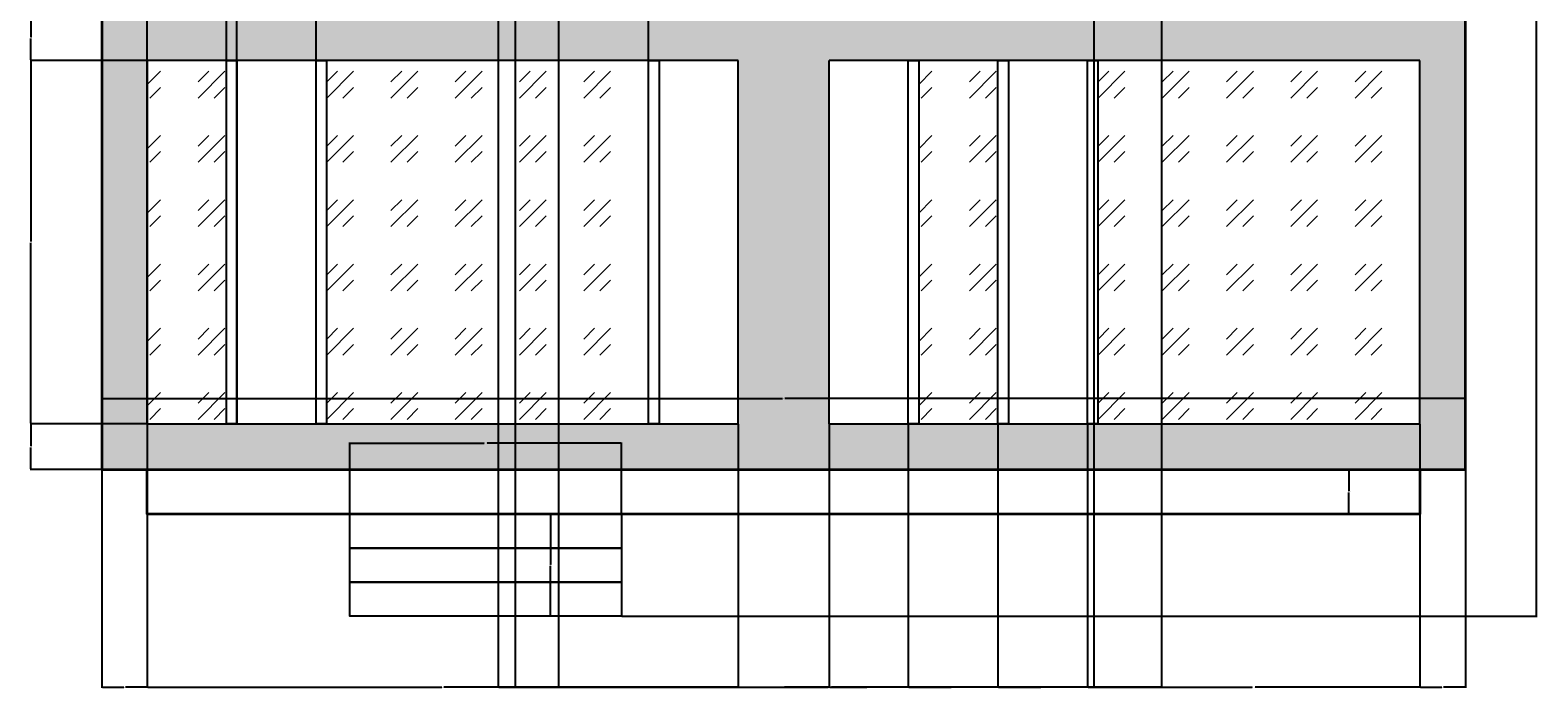
# Model space of a CAD drawing. Units: inches. Extents: x -9 to 389, y -55 to 344.
# Tile 1 of 5: x -9 to 389, y -55 to 119. Entities that reach past the tile are written whole.
import ezdxf

# ---------------------------------------------------------------- set-up
doc = ezdxf.new("R2010")
doc.units = ezdxf.units.IN
doc.header["$MEASUREMENT"] = 0
for name, color, linetype, lineweight in [('A-ANNO-DIMS', 2, 'Continuous', 18), ('A-ELEV', 7, 'Continuous', 35), ('A-ELEV-PATT', 8, 'Continuous', 13), ('A-FLOR-STRS', 3, 'Continuous', 25), ('A-GLAZ', 4, 'Continuous', 25), ('A-GLAZ-PATT', 252, 'Continuous', 13)]:
    doc.layers.add(name, color=color, linetype=linetype, lineweight=lineweight)
doc.styles.get("Standard").update_dxf_attribs({"font": 'arial.ttf'})
doc.dimstyles.get("Standard").update_dxf_attribs({"dimtxt": 0.18, "dimasz": 0.18, "dimexe": 0.18, "dimexo": 0.0625, "dimgap": 0.09, "dimtad": 0, "dimtih": 1, "dimtoh": 1, "dimdec": 4, "dimzin": 0, "dimdsep": 46, "dimtxsty": 'Standard', "dimcen": 0.09, "dimadec": 0, "dimazin": 0, "dimtfac": 1, "dimtdec": 4, "dimtofl": 0, "dimtmove": 0, "dimatfit": 3, "dimfxl": 1, "dimtolj": 1, "dimtzin": 0, "dimarcsym": 0})

# ---------------------------------------------------------------- blocks, each defined once
blk = doc.blocks.new('*D7')
at = {"layer": 'A-ANNO-DIMS', "color": 0, "lineweight": -2, "transparency": 16777216}
for p, q in [((9.65, 2.83), (9.65, 21.7)), ((9.83, 21.52), (189.36, 21.52)), ((369.47, 21.52), (189.94, 21.52)), ((369.65, 2.83), (369.65, 21.7))]:
    blk.add_line(p, q, dxfattribs=at)
at = {"layer": 'A-ANNO-DIMS', "color": 0, "transparency": 16777216}
for points in [[(9.83, 21.55), (9.83, 21.49), (9.65, 21.52)], [(369.47, 21.55), (369.47, 21.49), (369.65, 21.52)]]:
    blk.add_solid(points, dxfattribs=at)
at = {"layer": 'Defpoints', "color": 0, "transparency": 16777216}
for p in [(369.65, 21.52), (9.65, 2.77), (369.65, 2.77)]:
    blk.add_point(p, dxfattribs=at)
at = {"layer": 'A-ANNO-DIMS', "color": 0, "transparency": 16777216, "insert": (189.65, 21.52), "char_height": 0.18, "attachment_point": 5}
blk.add_mtext('\\A1;360', dxfattribs=at)
blk = doc.blocks.new('*D8')
at = {"layer": 'A-ANNO-DIMS', "color": 0, "lineweight": -2, "transparency": 16777216}
for p, q in [((21.65, 14.71), (21.65, -54.92)), ((9.65, 2.71), (9.65, -54.92)), ((9.83, -54.74), (15.44, -54.74)), ((21.47, -54.74), (15.86, -54.74))]:
    blk.add_line(p, q, dxfattribs=at)
at = {"layer": 'A-ANNO-DIMS', "color": 0, "transparency": 16777216}
for points in [[(9.83, -54.71), (9.83, -54.77), (9.65, -54.74)], [(21.47, -54.71), (21.47, -54.77), (21.65, -54.74)]]:
    blk.add_solid(points, dxfattribs=at)
at = {"layer": 'Defpoints', "color": 0, "transparency": 16777216}
for p in [(21.65, 14.77), (9.65, 2.77), (21.65, -54.74)]:
    blk.add_point(p, dxfattribs=at)
at = {"layer": 'A-ANNO-DIMS', "color": 0, "transparency": 16777216, "insert": (15.65, -54.74), "char_height": 0.18, "attachment_point": 5}
blk.add_mtext('\\A1;12', dxfattribs=at)
blk = doc.blocks.new('*D9')
at = {"layer": 'A-ANNO-DIMS', "color": 0, "lineweight": -2, "transparency": 16777216}
for p, q in [((21.65, 14.71), (21.65, -54.92)), ((177.65, 14.71), (177.65, -54.92)), ((21.83, -54.74), (99.37, -54.74)), ((177.47, -54.74), (99.93, -54.74))]:
    blk.add_line(p, q, dxfattribs=at)
at = {"layer": 'A-ANNO-DIMS', "color": 0, "transparency": 16777216}
for points in [[(21.83, -54.71), (21.83, -54.77), (21.65, -54.74)], [(177.47, -54.71), (177.47, -54.77), (177.65, -54.74)]]:
    blk.add_solid(points, dxfattribs=at)
at = {"layer": 'Defpoints', "color": 0, "transparency": 16777216}
for p in [(21.65, 14.77), (177.65, 14.77), (177.65, -54.74)]:
    blk.add_point(p, dxfattribs=at)
at = {"layer": 'A-ANNO-DIMS', "color": 0, "transparency": 16777216, "insert": (99.65, -54.74), "char_height": 0.18, "attachment_point": 5}
blk.add_mtext('\\A1;156', dxfattribs=at)
blk = doc.blocks.new('*D10')
at = {"layer": 'A-ANNO-DIMS', "color": 0, "lineweight": -2, "transparency": 16777216}
for p, q in [((177.65, 14.71), (177.65, -54.92)), ((201.65, 14.71), (201.65, -54.92)), ((177.83, -54.74), (189.43, -54.74)), ((201.47, -54.74), (189.87, -54.74))]:
    blk.add_line(p, q, dxfattribs=at)
at = {"layer": 'A-ANNO-DIMS', "color": 0, "transparency": 16777216}
for points in [[(177.83, -54.71), (177.83, -54.77), (177.65, -54.74)], [(201.47, -54.71), (201.47, -54.77), (201.65, -54.74)]]:
    blk.add_solid(points, dxfattribs=at)
at = {"layer": 'Defpoints', "color": 0, "transparency": 16777216}
for p in [(177.65, 14.77), (201.65, 14.77), (201.65, -54.74)]:
    blk.add_point(p, dxfattribs=at)
at = {"layer": 'A-ANNO-DIMS', "color": 0, "transparency": 16777216, "insert": (189.65, -54.74), "char_height": 0.18, "attachment_point": 5}
blk.add_mtext('\\A1;24', dxfattribs=at)
blk = doc.blocks.new('*D11')
at = {"layer": 'A-ANNO-DIMS', "color": 0, "lineweight": -2, "transparency": 16777216}
for p, q in [((201.65, 14.71), (201.65, -54.92)), ((222.55, 14.71), (222.55, -54.92)), ((201.83, -54.74), (211.64, -54.74)), ((222.37, -54.74), (212.57, -54.74))]:
    blk.add_line(p, q, dxfattribs=at)
at = {"layer": 'A-ANNO-DIMS', "color": 0, "transparency": 16777216}
for points in [[(201.83, -54.71), (201.83, -54.77), (201.65, -54.74)], [(222.37, -54.71), (222.37, -54.77), (222.55, -54.74)]]:
    blk.add_solid(points, dxfattribs=at)
at = {"layer": 'Defpoints', "color": 0, "transparency": 16777216}
for p in [(201.65, 14.77), (222.55, 14.77), (222.55, -54.74)]:
    blk.add_point(p, dxfattribs=at)
at = {"layer": 'A-ANNO-DIMS', "color": 0, "transparency": 16777216, "insert": (212.1, -54.74), "char_height": 0.18, "attachment_point": 5}
blk.add_mtext('\\A1;20.896', dxfattribs=at)
blk = doc.blocks.new('*D12')
at = {"layer": 'A-ANNO-DIMS', "color": 0, "lineweight": -2, "transparency": 16777216}
for p, q in [((222.55, 14.71), (222.55, -54.92)), ((246.21, 14.71), (246.21, -54.92)), ((222.73, -54.74), (233.92, -54.74)), ((246.03, -54.74), (234.85, -54.74))]:
    blk.add_line(p, q, dxfattribs=at)
at = {"layer": 'A-ANNO-DIMS', "color": 0, "transparency": 16777216}
for points in [[(222.73, -54.71), (222.73, -54.77), (222.55, -54.74)], [(246.03, -54.71), (246.03, -54.77), (246.21, -54.74)]]:
    blk.add_solid(points, dxfattribs=at)
at = {"layer": 'Defpoints', "color": 0, "transparency": 16777216}
for p in [(222.55, 14.77), (246.21, 14.77), (246.21, -54.74)]:
    blk.add_point(p, dxfattribs=at)
at = {"layer": 'A-ANNO-DIMS', "color": 0, "transparency": 16777216, "insert": (234.38, -54.74), "char_height": 0.18, "attachment_point": 5}
blk.add_mtext('\\A1;23.666', dxfattribs=at)
blk = doc.blocks.new('*D13')
at = {"layer": 'A-ANNO-DIMS', "color": 0, "lineweight": -2, "transparency": 16777216}
for p, q in [((246.21, 14.71), (246.21, -54.92)), ((269.88, 14.71), (269.88, -54.92)), ((246.39, -54.74), (257.58, -54.74)), ((269.7, -54.74), (258.51, -54.74))]:
    blk.add_line(p, q, dxfattribs=at)
at = {"layer": 'A-ANNO-DIMS', "color": 0, "transparency": 16777216}
for points in [[(246.39, -54.71), (246.39, -54.77), (246.21, -54.74)], [(269.7, -54.71), (269.7, -54.77), (269.88, -54.74)]]:
    blk.add_solid(points, dxfattribs=at)
at = {"layer": 'Defpoints', "color": 0, "transparency": 16777216}
for p in [(246.21, 14.77), (269.88, 14.77), (269.88, -54.74)]:
    blk.add_point(p, dxfattribs=at)
at = {"layer": 'A-ANNO-DIMS', "color": 0, "transparency": 16777216, "insert": (258.05, -54.74), "char_height": 0.18, "attachment_point": 5}
blk.add_mtext('\\A1;23.666', dxfattribs=at)
blk = doc.blocks.new('*D14')
at = {"layer": 'A-ANNO-DIMS', "color": 0, "lineweight": -2, "transparency": 16777216}
for p, q in [((269.88, 14.71), (269.88, -54.92)), ((357.65, 14.71), (357.65, -54.92)), ((270.06, -54.74), (313.37, -54.74)), ((357.47, -54.74), (314.16, -54.74))]:
    blk.add_line(p, q, dxfattribs=at)
at = {"layer": 'A-ANNO-DIMS', "color": 0, "transparency": 16777216}
for points in [[(270.06, -54.71), (270.06, -54.77), (269.88, -54.74)], [(357.47, -54.71), (357.47, -54.77), (357.65, -54.74)]]:
    blk.add_solid(points, dxfattribs=at)
at = {"layer": 'Defpoints', "color": 0, "transparency": 16777216}
for p in [(269.88, 14.77), (357.65, 14.77), (357.65, -54.74)]:
    blk.add_point(p, dxfattribs=at)
at = {"layer": 'A-ANNO-DIMS', "color": 0, "transparency": 16777216, "insert": (313.77, -54.74), "char_height": 0.18, "attachment_point": 5}
blk.add_mtext('\\A1;87.77', dxfattribs=at)
blk = doc.blocks.new('*D15')
at = {"layer": 'A-ANNO-DIMS', "color": 0, "lineweight": -2, "transparency": 16777216}
for p, q in [((357.65, 14.71), (357.65, -54.92)), ((369.65, 2.71), (369.65, -54.92)), ((357.83, -54.74), (363.44, -54.74)), ((369.47, -54.74), (363.86, -54.74))]:
    blk.add_line(p, q, dxfattribs=at)
at = {"layer": 'A-ANNO-DIMS', "color": 0, "transparency": 16777216}
for points in [[(357.83, -54.71), (357.83, -54.77), (357.65, -54.74)], [(369.47, -54.71), (369.47, -54.77), (369.65, -54.74)]]:
    blk.add_solid(points, dxfattribs=at)
at = {"layer": 'Defpoints', "color": 0, "transparency": 16777216}
for p in [(357.65, 14.77), (369.65, 2.77), (369.65, -54.74)]:
    blk.add_point(p, dxfattribs=at)
at = {"layer": 'A-ANNO-DIMS', "color": 0, "transparency": 16777216, "insert": (363.65, -54.74), "char_height": 0.18, "attachment_point": 5}
blk.add_mtext('\\A1;12', dxfattribs=at)
blk = doc.blocks.new('*D16')
at = {"layer": 'A-ANNO-DIMS', "color": 0, "lineweight": -2, "transparency": 16777216}
for p, q in [((21.65, 14.83), (21.65, 343.8)), ((21.83, 343.62), (31.64, 343.62)), ((42.37, 343.62), (32.57, 343.62)), ((42.55, 14.83), (42.55, 343.8))]:
    blk.add_line(p, q, dxfattribs=at)
at = {"layer": 'A-ANNO-DIMS', "color": 0, "transparency": 16777216}
for points in [[(21.83, 343.65), (21.83, 343.59), (21.65, 343.62)], [(42.37, 343.65), (42.37, 343.59), (42.55, 343.62)]]:
    blk.add_solid(points, dxfattribs=at)
at = {"layer": 'Defpoints', "color": 0, "transparency": 16777216}
for p in [(42.55, 343.62), (21.65, 14.77), (42.55, 14.77)]:
    blk.add_point(p, dxfattribs=at)
at = {"layer": 'A-ANNO-DIMS', "color": 0, "transparency": 16777216, "insert": (32.1, 343.62), "char_height": 0.18, "attachment_point": 5}
blk.add_mtext('\\A1;20.896', dxfattribs=at)
blk = doc.blocks.new('*D17')
at = {"layer": 'A-ANNO-DIMS', "color": 0, "lineweight": -2, "transparency": 16777216}
for p, q in [((42.55, 14.83), (42.55, 343.8)), ((42.73, 343.62), (43.61, 343.62)), ((45.14, 343.62), (44.26, 343.62)), ((45.32, 14.83), (45.32, 343.8))]:
    blk.add_line(p, q, dxfattribs=at)
at = {"layer": 'A-ANNO-DIMS', "color": 0, "transparency": 16777216}
for points in [[(42.73, 343.65), (42.73, 343.59), (42.55, 343.62)], [(45.14, 343.65), (45.14, 343.59), (45.32, 343.62)]]:
    blk.add_solid(points, dxfattribs=at)
at = {"layer": 'Defpoints', "color": 0, "transparency": 16777216}
for p in [(45.32, 343.62), (42.55, 14.77), (45.32, 14.77)]:
    blk.add_point(p, dxfattribs=at)
at = {"layer": 'A-ANNO-DIMS', "color": 0, "transparency": 16777216, "insert": (43.93, 343.62), "char_height": 0.18, "attachment_point": 5}
blk.add_mtext('\\A1;2.77', dxfattribs=at)
blk = doc.blocks.new('*D18')
at = {"layer": 'A-ANNO-DIMS', "color": 0, "lineweight": -2, "transparency": 16777216}
for p, q in [((45.32, 14.83), (45.32, 343.8)), ((45.5, 343.62), (55.3, 343.62)), ((66.03, 343.62), (56.23, 343.62)), ((66.21, 14.83), (66.21, 343.8))]:
    blk.add_line(p, q, dxfattribs=at)
at = {"layer": 'A-ANNO-DIMS', "color": 0, "transparency": 16777216}
for points in [[(45.5, 343.65), (45.5, 343.59), (45.32, 343.62)], [(66.03, 343.65), (66.03, 343.59), (66.21, 343.62)]]:
    blk.add_solid(points, dxfattribs=at)
at = {"layer": 'Defpoints', "color": 0, "transparency": 16777216}
for p in [(66.21, 343.62), (45.32, 14.77), (66.21, 14.77)]:
    blk.add_point(p, dxfattribs=at)
at = {"layer": 'A-ANNO-DIMS', "color": 0, "transparency": 16777216, "insert": (55.77, 343.62), "char_height": 0.18, "attachment_point": 5}
blk.add_mtext('\\A1;20.896', dxfattribs=at)
blk = doc.blocks.new('*D19')
at = {"layer": 'A-ANNO-DIMS', "color": 0, "lineweight": -2, "transparency": 16777216}
for p, q in [((66.21, 14.83), (66.21, 343.8)), ((66.39, 343.62), (109.71, 343.62)), ((153.81, 343.62), (110.5, 343.62)), ((153.99, 14.83), (153.99, 343.8))]:
    blk.add_line(p, q, dxfattribs=at)
at = {"layer": 'A-ANNO-DIMS', "color": 0, "transparency": 16777216}
for points in [[(66.39, 343.65), (66.39, 343.59), (66.21, 343.62)], [(153.81, 343.65), (153.81, 343.59), (153.99, 343.62)]]:
    blk.add_solid(points, dxfattribs=at)
at = {"layer": 'Defpoints', "color": 0, "transparency": 16777216}
for p in [(153.99, 343.62), (66.21, 14.77), (153.99, 14.77)]:
    blk.add_point(p, dxfattribs=at)
at = {"layer": 'A-ANNO-DIMS', "color": 0, "transparency": 16777216, "insert": (110.1, 343.62), "char_height": 0.18, "attachment_point": 5}
blk.add_mtext('\\A1;87.77', dxfattribs=at)
blk = doc.blocks.new('*D20')
at = {"layer": 'A-ANNO-DIMS', "color": 0, "lineweight": -2, "transparency": 16777216}
for p, q in [((369.72, 324.87), (388.58, 324.87)), ((388.4, 324.69), (388.4, 144.62)), ((388.4, -35.81), (388.4, 144.26)), ((146.92, -35.99), (388.58, -35.99))]:
    blk.add_line(p, q, dxfattribs=at)
at = {"layer": 'A-ANNO-DIMS', "color": 0, "transparency": 16777216}
for points in [[(388.37, 324.69), (388.43, 324.69), (388.4, 324.87)], [(388.37, -35.81), (388.43, -35.81), (388.4, -35.99)]]:
    blk.add_solid(points, dxfattribs=at)
at = {"layer": 'Defpoints', "color": 0, "transparency": 16777216}
for p in [(369.65, 324.87), (388.4, 324.87), (146.86, -35.99)]:
    blk.add_point(p, dxfattribs=at)
at = {"layer": 'A-ANNO-DIMS', "color": 0, "transparency": 16777216, "insert": (388.4, 144.44), "char_height": 0.18, "attachment_point": 5}
blk.add_mtext('\\A1;360.86', dxfattribs=at)
blk = doc.blocks.new('*D21')
at = {"layer": 'A-ANNO-DIMS', "color": 0, "lineweight": -2, "transparency": 16777216}
for p, q in [((21.59, 14.77), (-9.28, 14.77)), ((-9.1, 14.59), (-9.1, 8.95)), ((-9.1, 2.95), (-9.1, 8.59)), ((9.59, 2.77), (-9.28, 2.77))]:
    blk.add_line(p, q, dxfattribs=at)
at = {"layer": 'A-ANNO-DIMS', "color": 0, "transparency": 16777216}
for points in [[(-9.13, 14.59), (-9.07, 14.59), (-9.1, 14.77)], [(-9.13, 2.95), (-9.07, 2.95), (-9.1, 2.77)]]:
    blk.add_solid(points, dxfattribs=at)
at = {"layer": 'Defpoints', "color": 0, "transparency": 16777216}
for p in [(-9.1, 14.77), (21.65, 14.77), (9.65, 2.77)]:
    blk.add_point(p, dxfattribs=at)
at = {"layer": 'A-ANNO-DIMS', "color": 0, "transparency": 16777216, "insert": (-9.1, 8.77), "char_height": 0.18, "attachment_point": 5}
blk.add_mtext('\\A1;12', dxfattribs=at)
blk = doc.blocks.new('*D22')
at = {"layer": 'A-ANNO-DIMS', "color": 0, "lineweight": -2, "transparency": 16777216}
for p, q in [((21.59, 110.77), (-9.28, 110.77)), ((-9.1, 110.59), (-9.1, 62.95)), ((-9.1, 14.95), (-9.1, 62.59)), ((21.59, 14.77), (-9.28, 14.77))]:
    blk.add_line(p, q, dxfattribs=at)
at = {"layer": 'A-ANNO-DIMS', "color": 0, "transparency": 16777216}
for points in [[(-9.13, 110.59), (-9.07, 110.59), (-9.1, 110.77)], [(-9.13, 14.95), (-9.07, 14.95), (-9.1, 14.77)]]:
    blk.add_solid(points, dxfattribs=at)
at = {"layer": 'Defpoints', "color": 0, "transparency": 16777216}
for p in [(-9.1, 110.77), (21.65, 110.77), (21.65, 14.77)]:
    blk.add_point(p, dxfattribs=at)
at = {"layer": 'A-ANNO-DIMS', "color": 0, "transparency": 16777216, "insert": (-9.1, 62.77), "char_height": 0.18, "attachment_point": 5}
blk.add_mtext('\\A1;96', dxfattribs=at)
blk = doc.blocks.new('*D23')
at = {"layer": 'A-ANNO-DIMS', "color": 0, "lineweight": -2, "transparency": 16777216}
for p, q in [((9.59, 122.77), (-9.28, 122.77)), ((-9.1, 122.59), (-9.1, 116.95)), ((-9.1, 110.95), (-9.1, 116.59)), ((21.59, 110.77), (-9.28, 110.77))]:
    blk.add_line(p, q, dxfattribs=at)
at = {"layer": 'A-ANNO-DIMS', "color": 0, "transparency": 16777216}
for points in [[(-9.13, 122.59), (-9.07, 122.59), (-9.1, 122.77)], [(-9.13, 110.95), (-9.07, 110.95), (-9.1, 110.77)]]:
    blk.add_solid(points, dxfattribs=at)
at = {"layer": 'Defpoints', "color": 0, "transparency": 16777216}
for p in [(-9.1, 122.77), (9.65, 122.77), (21.65, 110.77)]:
    blk.add_point(p, dxfattribs=at)
at = {"layer": 'A-ANNO-DIMS', "color": 0, "transparency": 16777216, "insert": (-9.1, 116.77), "char_height": 0.18, "attachment_point": 5}
blk.add_mtext('\\A1;12', dxfattribs=at)
blk = doc.blocks.new('*D30')
at = {"layer": 'A-ANNO-DIMS', "color": 0, "lineweight": -2, "transparency": 16777216}
for p, q in [((146.8, -9.03), (127.93, -9.03)), ((128.11, -9.21), (128.11, -22.33)), ((128.11, -35.81), (128.11, -22.69)), ((146.8, -35.99), (127.93, -35.99))]:
    blk.add_line(p, q, dxfattribs=at)
at = {"layer": 'A-ANNO-DIMS', "color": 0, "transparency": 16777216}
for points in [[(128.08, -9.21), (128.14, -9.21), (128.11, -9.03)], [(128.08, -35.81), (128.14, -35.81), (128.11, -35.99)]]:
    blk.add_solid(points, dxfattribs=at)
at = {"layer": 'Defpoints', "color": 0, "transparency": 16777216}
for p in [(128.11, -9.03), (146.86, -9.03), (146.86, -35.99)]:
    blk.add_point(p, dxfattribs=at)
at = {"layer": 'A-ANNO-DIMS', "color": 0, "transparency": 16777216, "insert": (128.11, -22.51), "char_height": 0.18, "attachment_point": 5}
blk.add_mtext('\\A1;26.96', dxfattribs=at)
blk = doc.blocks.new('*D31')
at = {"layer": 'A-ANNO-DIMS', "color": 0, "lineweight": -2, "transparency": 16777216}
for p, q in [((357.59, 2.77), (338.72, 2.77)), ((338.9, 2.59), (338.9, -2.95)), ((338.9, -8.85), (338.9, -3.31)), ((357.59, -9.03), (338.72, -9.03))]:
    blk.add_line(p, q, dxfattribs=at)
at = {"layer": 'A-ANNO-DIMS', "color": 0, "transparency": 16777216}
for points in [[(338.87, 2.59), (338.93, 2.59), (338.9, 2.77)], [(338.87, -8.85), (338.93, -8.85), (338.9, -9.03)]]:
    blk.add_solid(points, dxfattribs=at)
at = {"layer": 'Defpoints', "color": 0, "transparency": 16777216}
for p in [(338.9, 2.77), (357.65, 2.77), (357.65, -9.03)]:
    blk.add_point(p, dxfattribs=at)
at = {"layer": 'A-ANNO-DIMS', "color": 0, "transparency": 16777216, "insert": (338.9, -3.13), "char_height": 0.18, "attachment_point": 5}
blk.add_mtext('\\A1;11.798', dxfattribs=at)
blk = doc.blocks.new('*D36')
at = {"layer": 'A-ANNO-DIMS', "color": 0, "lineweight": -2, "transparency": 16777216}
for p, q in [((75.15, -8.97), (75.15, 9.9)), ((75.33, 9.72), (110.63, 9.72)), ((146.68, 9.72), (111.38, 9.72)), ((146.86, -8.97), (146.86, 9.9))]:
    blk.add_line(p, q, dxfattribs=at)
at = {"layer": 'A-ANNO-DIMS', "color": 0, "transparency": 16777216}
for points in [[(75.33, 9.75), (75.33, 9.69), (75.15, 9.72)], [(146.68, 9.75), (146.68, 9.69), (146.86, 9.72)]]:
    blk.add_solid(points, dxfattribs=at)
at = {"layer": 'Defpoints', "color": 0, "transparency": 16777216}
for p in [(146.86, 9.72), (75.15, -9.03), (146.86, -9.03)]:
    blk.add_point(p, dxfattribs=at)
at = {"layer": 'A-ANNO-DIMS', "color": 0, "transparency": 16777216, "insert": (111.01, 9.72), "char_height": 0.18, "attachment_point": 5}
blk.add_mtext('\\A1;71.71', dxfattribs=at)
blk = doc.blocks.new('*D65')
at = {"layer": 'A-ANNO-DIMS', "color": 0, "lineweight": -2, "transparency": 16777216}
for p, q in [((130.2, 126.68), (130.2, -54.92)), ((118.78, 122.71), (118.78, -54.92)), ((118.96, -54.74), (124.11, -54.74)), ((130.02, -54.74), (124.88, -54.74))]:
    blk.add_line(p, q, dxfattribs=at)
at = {"layer": 'A-ANNO-DIMS', "color": 0, "transparency": 16777216}
for points in [[(118.96, -54.71), (118.96, -54.77), (118.78, -54.74)], [(130.02, -54.71), (130.02, -54.77), (130.2, -54.74)]]:
    blk.add_solid(points, dxfattribs=at)
at = {"layer": 'Defpoints', "color": 0, "transparency": 16777216}
for p in [(130.2, 126.74), (118.78, 122.77), (130.2, -54.74)]:
    blk.add_point(p, dxfattribs=at)
at = {"layer": 'A-ANNO-DIMS', "color": 0, "transparency": 16777216, "insert": (124.49, -54.74), "char_height": 0.18, "attachment_point": 5}
blk.add_mtext('\\A1;11.42', dxfattribs=at)
blk = doc.blocks.new('*D67')
at = {"layer": 'A-ANNO-DIMS', "color": 0, "lineweight": -2, "transparency": 16777216}
for p, q in [((271.58, 128.99), (271.58, -54.92)), ((289.4, 122.71), (289.4, -54.92)), ((271.76, -54.74), (280.03, -54.74)), ((289.22, -54.74), (280.94, -54.74))]:
    blk.add_line(p, q, dxfattribs=at)
at = {"layer": 'A-ANNO-DIMS', "color": 0, "transparency": 16777216}
for points in [[(271.76, -54.71), (271.76, -54.77), (271.58, -54.74)], [(289.22, -54.71), (289.22, -54.77), (289.4, -54.74)]]:
    blk.add_solid(points, dxfattribs=at)
at = {"layer": 'Defpoints', "color": 0, "transparency": 16777216}
for p in [(271.58, 129.05), (289.4, 122.77), (289.4, -54.74)]:
    blk.add_point(p, dxfattribs=at)
at = {"layer": 'A-ANNO-DIMS', "color": 0, "transparency": 16777216, "insert": (280.49, -54.74), "char_height": 0.18, "attachment_point": 5}
blk.add_mtext('\\A1;17.817', dxfattribs=at)
blk = doc.blocks.new('*D68')
at = {"layer": 'A-ANNO-DIMS', "color": 0, "lineweight": -2, "transparency": 16777216}
for p, q in [((114.32, 122.71), (114.32, -54.92)), ((289.4, 122.71), (289.4, -54.92)), ((114.5, -54.74), (201.4, -54.74)), ((289.22, -54.74), (202.31, -54.74))]:
    blk.add_line(p, q, dxfattribs=at)
at = {"layer": 'A-ANNO-DIMS', "color": 0, "transparency": 16777216}
for points in [[(114.5, -54.71), (114.5, -54.77), (114.32, -54.74)], [(289.22, -54.71), (289.22, -54.77), (289.4, -54.74)]]:
    blk.add_solid(points, dxfattribs=at)
at = {"layer": 'Defpoints', "color": 0, "transparency": 16777216}
for p in [(114.32, 122.77), (289.4, 122.77), (289.4, -54.74)]:
    blk.add_point(p, dxfattribs=at)
at = {"layer": 'A-ANNO-DIMS', "color": 0, "transparency": 16777216, "insert": (201.86, -54.74), "char_height": 0.18, "attachment_point": 5}
blk.add_mtext('\\A1;175.08', dxfattribs=at)

msp = doc.modelspace()

# ---------------------------------------------------------------- hatches: boundary and pattern name
at = {"layer": 'A-ELEV-PATT'}
h = msp.add_hatch(color=256, dxfattribs=at)
h.dxf.hatch_style = 1
h.paths.add_polyline_path([(369.6533, 122.7681), (289.3963, 122.7681), (9.6533, 122.7681), (9.6533, 2.7681), (369.6533, 2.7681)])
h.paths.add_polyline_path([(177.6533, 110.7681), (177.6533, 14.7681), (21.6533, 14.7681), (21.6533, 110.7681)], flags=16)
h.paths.add_polyline_path([(201.6533, 110.7681), (357.6533, 110.7681), (357.6533, 14.7681), (201.6533, 14.7681)], flags=16)
h.paths.add_polyline_path([(156.7573, 110.7681), (156.7573, 14.7681), (153.9877, 14.7681), (153.9877, 110.7681)], flags=0)
h.paths.add_polyline_path([(222.5492, 110.7681), (225.3188, 110.7681), (225.3188, 14.7681), (222.5492, 14.7681)], flags=0)
h.paths.add_polyline_path([(246.2148, 110.7681), (248.9844, 110.7681), (248.9844, 14.7681), (246.2148, 14.7681)], flags=0)
h.paths.add_polyline_path([(269.8803, 110.7681), (272.65, 110.7681), (272.65, 14.7681), (269.8803, 14.7681)], flags=0)
h.paths.add_polyline_path([(68.9844, 110.7681), (68.9844, 14.7681), (66.2148, 14.7681), (66.2148, 110.7681)], flags=0)
h.paths.add_polyline_path([(45.3188, 110.7681), (45.3188, 14.7681), (42.5492, 14.7681), (42.5492, 110.7681)], flags=0)
at = {"layer": 'A-GLAZ-PATT', "transparency": 33554536}
h = msp.add_hatch(dxfattribs=at)
h.set_pattern_fill('GOST_GLASS', color=256, scale=2)
h.set_pattern_definition([(45, (-83.729, -34.93), (16.97056, 0), [10, -14]), (45, (-79.486, -34.93), (16.97056, 0), [4, -20]), (45, (-83.729, -30.687), (16.97056, 0), [4, -20])])
h.paths.add_polyline_path([(153.9877, 110.7681), (68.9844, 110.7681), (68.9844, 14.7681), (153.9877, 14.7681)])
h.paths.add_polyline_path([(357.6533, 110.7681), (272.65, 110.7681), (272.65, 14.7681), (357.6533, 14.7681)])
h.paths.add_polyline_path([(190.6266, 218.7681), (169.7307, 218.7681), (169.7307, 146.7681), (190.6266, 146.7681)])
h.paths.add_polyline_path([(143.2954, 218.7681), (122.3995, 218.7681), (122.3995, 146.7681), (143.2954, 146.7681)])
h.paths.add_polyline_path([(237.9578, 184.6816), (217.3576, 218.7681), (217.0618, 218.7681), (217.0618, 146.7681), (237.9578, 146.7681)])
h.paths.add_polyline_path([(42.5492, 110.7681), (21.6533, 110.7681), (21.6533, 14.7681), (42.5492, 14.7681)])
h.paths.add_polyline_path([(246.2148, 110.7681), (225.3188, 110.7681), (225.3188, 14.7681), (246.2148, 14.7681)])

# ---------------------------------------------------------------- linework, layer by layer
at = {"layer": 'A-ELEV'}
for p, q in [((9.6533, 242.7681), (9.6533, 2.7681)), ((369.6533, 2.7681), (369.6533, 242.7681)), ((9.6533, 2.7681), (369.6533, 2.7681))]:
    msp.add_line(p, q, dxfattribs=at)
msp.add_lwpolyline([(21.6533, 2.7681), (357.6533, 2.7681), (357.6533, -9.0302), (21.6533, -9.0302)], close=True, dxfattribs=at)
at = {"layer": 'A-FLOR-STRS'}
for points in [[(75.1501, -9.0302), (146.8603, -9.0302), (146.8603, -18.0163), (75.1501, -18.0163)], [(75.1501, -18.0163), (146.8603, -18.0163), (146.8603, -27.0024), (75.1501, -27.0024)], [(75.1501, -27.0024), (146.8603, -27.0024), (146.8603, -35.9886), (75.1501, -35.9886)]]:
    msp.add_lwpolyline(points, close=True, dxfattribs=at)
at = {"layer": 'A-GLAZ'}
for p, q in [((21.6533, 110.7681), (21.6533, 14.7681)), ((177.6533, 110.7681), (21.6533, 110.7681)), ((177.6533, 14.7681), (177.6533, 110.7681)), ((357.6533, 110.7681), (201.6533, 110.7681)), ((201.6533, 14.7681), (201.6533, 110.7681)), ((357.6533, 14.7681), (357.6533, 110.7681)), ((21.6533, 14.7681), (177.6533, 14.7681)), ((201.6533, 14.7681), (357.6533, 14.7681))]:
    msp.add_line(p, q, dxfattribs=at)
for points in [[(42.5492, 110.7681), (45.3188, 110.7681), (45.3188, 14.7681), (42.5492, 14.7681)], [(66.2148, 110.7681), (68.9844, 110.7681), (68.9844, 14.7681), (66.2148, 14.7681)], [(153.9877, 110.7681), (156.7573, 110.7681), (156.7573, 14.7681), (153.9877, 14.7681)], [(222.5492, 110.7681), (225.3188, 110.7681), (225.3188, 14.7681), (222.5492, 14.7681)], [(246.2148, 110.7681), (248.9844, 110.7681), (248.9844, 14.7681), (246.2148, 14.7681)], [(269.8803, 110.7681), (272.65, 110.7681), (272.65, 14.7681), (269.8803, 14.7681)]]:
    msp.add_lwpolyline(points, close=True, dxfattribs=at)

# ---------------------------------------------------------------- dimensions: what is measured, and where the dimension line sits
at = {"layer": 'A-ANNO-DIMS'}
for base, p1, p2, override, picture, middle in [((42.5492, 343.6213), (21.6533, 14.7681), (42.5492, 14.7681), {"dimdec": 3, "dimlfac": 1, "dimrnd": 0, "dimzin": 0, "dimdsep": 46, "dimlunit": 2}, '*D16', (32.1012, 343.6213)), ((45.3188, 343.6213), (42.5492, 14.7681), (45.3188, 14.7681), {"dimdec": 2, "dimlfac": 1, "dimrnd": 0, "dimzin": 0, "dimdsep": 46, "dimlunit": 2}, '*D17', (43.934, 343.6213)), ((66.2148, 343.6213), (45.3188, 14.7681), (66.2148, 14.7681), {"dimdec": 3, "dimlfac": 1, "dimrnd": 0, "dimzin": 0, "dimdsep": 46, "dimlunit": 2}, '*D18', (55.7668, 343.6213)), ((153.9877, 343.6213), (66.2148, 14.7681), (153.9877, 14.7681), {"dimdec": 2, "dimlfac": 1, "dimrnd": 0, "dimzin": 0, "dimdsep": 46, "dimlunit": 2}, '*D19', (110.1012, 343.6213)), ((289.3963, -54.7386), (271.5791, 129.0492), (289.3963, 122.7681), {"dimdec": 3, "dimlfac": 1, "dimrnd": 0, "dimzin": 0, "dimdsep": 46, "dimlunit": 2}, '*D67', (280.4877, -54.7386)), ((130.2035, -54.7386), (118.7824, 122.7681), (130.2035, 126.7437), {"dimdec": 2, "dimlfac": 1, "dimrnd": 0, "dimzin": 0, "dimdsep": 46, "dimlunit": 2}, '*D65', (124.493, -54.7386)), ((289.3963, -54.7386), (114.32, 122.7681), (289.3963, 122.7681), {"dimdec": 2, "dimlfac": 1, "dimrnd": 0, "dimzin": 0, "dimdsep": 46, "dimlunit": 2}, '*D68', (201.8582, -54.7386)), ((369.6533, 21.5181), (9.6533, 2.7681), (369.6533, 2.7681), {"dimdec": 0, "dimlfac": 1, "dimrnd": 0, "dimzin": 0, "dimdsep": 46, "dimlunit": 2}, '*D7', (189.6533, 21.5181)), ((21.6533, -54.7386), (9.6533, 2.7681), (21.6533, 14.7681), {"dimdec": 0, "dimlfac": 1, "dimrnd": 0, "dimzin": 0, "dimdsep": 46, "dimlunit": 2}, '*D8', (15.6533, -54.7386)), ((177.6533, -54.7386), (21.6533, 14.7681), (177.6533, 14.7681), {"dimdec": 0, "dimlfac": 1, "dimrnd": 0, "dimzin": 0, "dimdsep": 46, "dimlunit": 2}, '*D9', (99.6533, -54.7386)), ((201.6533, -54.7386), (177.6533, 14.7681), (201.6533, 14.7681), {"dimdec": 0, "dimlfac": 1, "dimrnd": 0, "dimzin": 0, "dimdsep": 46, "dimlunit": 2}, '*D10', (189.6533, -54.7386)), ((222.5492, -54.7386), (201.6533, 14.7681), (222.5492, 14.7681), {"dimdec": 3, "dimlfac": 1, "dimrnd": 0, "dimzin": 0, "dimdsep": 46, "dimlunit": 2}, '*D11', (212.1012, -54.7386)), ((246.2148, -54.7386), (222.5492, 14.7681), (246.2148, 14.7681), {"dimdec": 3, "dimlfac": 1, "dimrnd": 0, "dimzin": 0, "dimdsep": 46, "dimlunit": 2}, '*D12', (234.382, -54.7386)), ((269.88034, -54.73859), (246.21476, 14.76811), (269.88034, 14.76811), {"dimdec": 3, "dimlfac": 1, "dimrnd": 0, "dimzin": 0, "dimdsep": 46, "dimlunit": 2}, '*D13', (258.04755, -54.73859)), ((357.6533, -54.7386), (269.8803, 14.7681), (357.6533, 14.7681), {"dimdec": 2, "dimlfac": 1, "dimrnd": 0, "dimzin": 0, "dimdsep": 46, "dimlunit": 2}, '*D14', (313.7668, -54.7386)), ((369.6533, -54.7386), (357.6533, 14.7681), (369.6533, 2.7681), {"dimdec": 0, "dimlfac": 1, "dimrnd": 0, "dimzin": 0, "dimdsep": 46, "dimlunit": 2}, '*D15', (363.6533, -54.7386)), ((146.8603, 9.7198), (75.1501, -9.0302), (146.8603, -9.0302), {"dimdec": 2, "dimlfac": 1, "dimrnd": 0, "dimzin": 0, "dimdsep": 46, "dimlunit": 2}, '*D36', (111.0052, 9.7198))]:
    dim = msp.add_linear_dim(base=base, p1=p1, p2=p2, dimstyle='Standard', override=override, dxfattribs=at)
    dim.commit()
    dim.dimension.update_dxf_attribs({"geometry": picture, "text_midpoint": middle})
for base, p1, p2, override, picture, middle in [((388.4033, 324.8713), (146.8603, -35.9886), (369.6533, 324.8713), {"dimdec": 2, "dimlfac": 1, "dimrnd": 0, "dimzin": 0, "dimdsep": 46, "dimlunit": 2}, '*D20', (388.4033, 144.4414)), ((-9.0967, 122.7681), (21.6533, 110.7681), (9.6533, 122.7681), {"dimdec": 0, "dimlfac": 1, "dimrnd": 0, "dimzin": 0, "dimdsep": 46, "dimlunit": 2}, '*D23', (-9.0967, 116.7681)), ((-9.0967, 110.7681), (21.6533, 14.7681), (21.6533, 110.7681), {"dimdec": 0, "dimlfac": 1, "dimrnd": 0, "dimzin": 0, "dimdsep": 46, "dimlunit": 2}, '*D22', (-9.0967, 62.7681)), ((-9.0967, 14.7681), (9.6533, 2.7681), (21.6533, 14.7681), {"dimdec": 0, "dimlfac": 1, "dimrnd": 0, "dimzin": 0, "dimdsep": 46, "dimlunit": 2}, '*D21', (-9.0967, 8.7681)), ((338.9033, 2.7681), (357.6533, -9.0302), (357.6533, 2.7681), {"dimdec": 3, "dimlfac": 1, "dimrnd": 0, "dimzin": 0, "dimdsep": 46, "dimlunit": 2}, '*D31', (338.9033, -3.131)), ((128.1103, -9.0302), (146.8603, -35.9886), (146.8603, -9.0302), {"dimdec": 2, "dimlfac": 1, "dimrnd": 0, "dimzin": 0, "dimdsep": 46, "dimlunit": 2}, '*D30', (128.1103, -22.5094))]:
    dim = msp.add_linear_dim(base=base, p1=p1, p2=p2, angle=90, dimstyle='Standard', override=override, dxfattribs=at)
    dim.commit()
    dim.dimension.update_dxf_attribs({"geometry": picture, "text_midpoint": middle})

doc.saveas('drawing.dxf')
